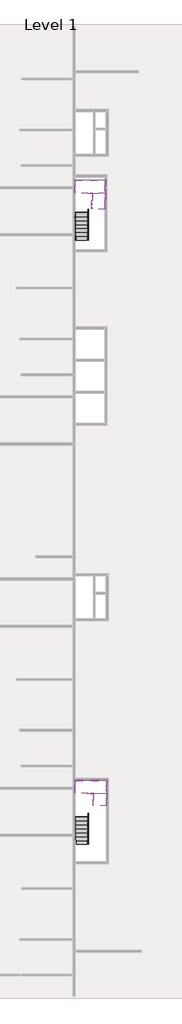
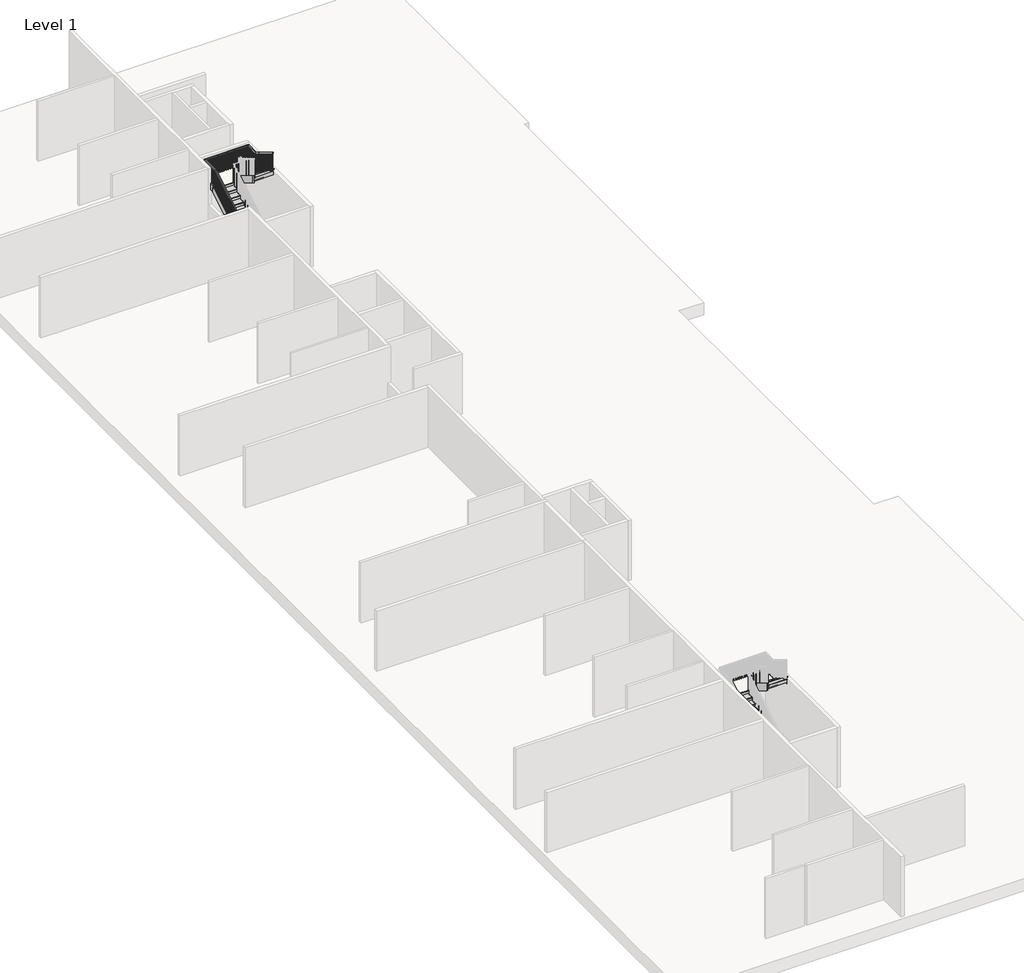
# One storey, part 8 of 8: 16 members, 4 stair flights, 2 slabs, 1 railing.
"""IFC4 building model written with IfcOpenShell, lengths in millimetres."""

from ifc_helpers import new_model, si_unit, frame, origin, place, context, project, spatial, polyline, outline, extrude, faceted_brep, transform, mapped, element, save
from components import non_monolithic_landing_1722db8f, non_monolithic_landing_351a0d85, stair_flight_df872bfd, stair_flight_7c360194, stair_flight_c0f4d4ee, stair_flight_213872ae

model = new_model("IFC4")

# Units and contexts
model_context = context("Model", 3, world=origin())
ifc_project = project(units=[si_unit("LENGTHUNIT", "METRE", prefix="MILLI")], contexts=[model_context])

# Site, building, storey
site = spatial("IfcSite", under=ifc_project)
building = spatial("IfcBuilding", under=site)
storey = spatial("IfcBuildingStorey", under=building, Name="Level 1", Elevation=25234.6172466)

# Members
placement = place(None, origin())
element("IfcMember", 1, ObjectType="Stringer - 2\" Width", at=placement, inside=storey, context=model_context, shape_type="SweptSolid", body=[
    extrude(outline(polyline([(-23154.3851539, 25234.6172466), (-23154.3851539, 25446.7317586), (-19467.0440987, 27681.4839133), (-19381.8896422, 27376.6839133), (-22916.2996422, 25234.6172466), (-23154.3851539, 25234.6172466)])), frame((-3668.2415084, 0.0, 0.0), z_axis=(1.0, 0.0, 0.0), x_axis=(0.0, 1.0, 0.0)), (0.0, 0.0, 1.0), 50.8),
])
element("IfcMember", 2, ObjectType="Stringer - 2\" Width", at=placement, inside=storey, context=model_context, shape_type="SweptSolid", body=[
    extrude(outline(polyline([(-23154.3851539, 25234.6172466), (-23154.3851539, 25446.7317586), (-19572.9851539, 27617.2772131), (-19572.9851539, 27260.8684516), (-22916.2996422, 25234.6172466), (-23154.3851539, 25234.6172466)])), frame((-2703.0415084, 0.0, 0.0), z_axis=(1.0, 0.0, 0.0), x_axis=(0.0, 1.0, 0.0)), (0.0, 0.0, 1.0), 50.8),
])
element("IfcMember", 3, ObjectType="Stringer - 2\" Width", at=placement, inside=storey, context=model_context, shape_type="SweptSolid", body=[
    extrude(outline(polyline([(-19297.9262092, 27681.4839133), (-19383.0806657, 27376.6839133), (-20360.3851539, 27968.9896637), (-20360.3851539, 28325.3984252), (-19297.9262092, 27681.4839133)])), frame((-1382.2415084, 0.0, 0.0), z_axis=(1.0, 0.0, 0.0), x_axis=(0.0, 1.0, 0.0)), (0.0, 0.0, 1.0), 50.8),
])
element("IfcMember", 4, ObjectType="Stringer - 2\" Width", at=placement, inside=storey, context=model_context, shape_type="SweptSolid", body=[
    extrude(outline(polyline([(-19522.1851539, 27817.3984252), (-19522.1851539, 27460.9896637), (-20360.3851539, 27968.9896637), (-20360.3851539, 28325.3984252), (-19522.1851539, 27817.3984252)])), frame((-2347.4415084, 0.0, 0.0), z_axis=(1.0, 0.0, 0.0), x_axis=(0.0, 1.0, 0.0)), (0.0, 0.0, 1.0), 50.8),
])
element("IfcMember", 5, ObjectType="Stringer - 2\" Width", at=placement, inside=storey, context=model_context, shape_type="Brep", body=[
    faceted_brep([(-1382.2415084, -19297.9262092, 27681.4839133), (-1331.4415084, -19297.9262092, 27681.4839133), (-1331.4415084, -18556.9851539, 27681.4839133), (-1382.2415084, -18607.7851539, 27681.4839133), (-1382.2415084, -19383.0806657, 27376.6839133), (-1382.2415084, -18607.7851539, 27376.6839133), (-1331.4415084, -19383.0806657, 27376.6839133), (-1331.4415084, -18556.9851539, 27376.6839133)], [[[0, 1, 2, 3]], [[4, 0, 3, 5]], [[6, 4, 5, 7]], [[1, 6, 7, 2]], [[1, 0, 4, 6]], [[2, 7, 5, 3]]]),
])
element("IfcMember", 6, ObjectType="Stringer - 2\" Width", at=placement, inside=storey, context=model_context, shape_type="SweptSolid", body=[
    extrude(outline(polyline([(-1331.4415084, -18556.9851539), (-1382.2415084, -18607.7851539), (-3617.4415084, -18607.7851539), (-3668.2415084, -18556.9851539), (-1331.4415084, -18556.9851539)])), frame((0.0, 0.0, 27376.6839133), z_axis=(0.0, 0.0, 1.0), x_axis=(1.0, 0.0, 0.0)), (0.0, 0.0, 1.0), 304.8),
])
element("IfcMember", 7, ObjectType="Stringer - 2\" Width", at=placement, inside=storey, context=model_context, shape_type="Brep", body=[
    faceted_brep([(-3617.4415084, -18607.7851539, 27681.4839133), (-3668.2415084, -18556.9851539, 27681.4839133), (-3668.2415084, -19467.0440987, 27681.4839133), (-3617.4415084, -19467.0440987, 27681.4839133), (-3617.4415084, -18607.7851539, 27376.6839133), (-3617.4415084, -19381.8896422, 27376.6839133), (-3668.2415084, -18556.9851539, 27376.6839133), (-3668.2415084, -19381.8896422, 27376.6839133)], [[[0, 1, 2, 3]], [[4, 0, 3, 5]], [[6, 4, 5, 7]], [[1, 6, 7, 2]], [[1, 0, 4, 6]], [[2, 7, 5, 3]]]),
])
element("IfcMember", 8, ObjectType="Stringer - 2\" Width", at=placement, inside=storey, context=model_context, shape_type="SweptSolid", body=[
    extrude(outline(polyline([(-2703.0415084, -19572.9851539), (-2703.0415084, -19522.1851539), (-2347.4415084, -19522.1851539), (-2347.4415084, -19572.9851539), (-2703.0415084, -19572.9851539)])), frame((0.0, 0.0, 27376.6839133), z_axis=(0.0, 0.0, 1.0), x_axis=(1.0, 0.0, 0.0)), (0.0, 0.0, 1.0), 304.8),
])
element("IfcMember", 9, ObjectType="Stringer - 2\" Width", at=placement, inside=storey, context=model_context, shape_type="SweptSolid", body=[
    extrude(outline(polyline([(19841.9216096, 25234.6172466), (19841.9216096, 25446.7317586), (23249.8626649, 27512.1505799), (23335.0171214, 27207.3505799), (20080.0071214, 25234.6172466), (19841.9216096, 25234.6172466)])), frame((-3668.2415084, 0.0, 0.0), z_axis=(1.0, 0.0, 0.0), x_axis=(0.0, 1.0, 0.0)), (0.0, 0.0, 1.0), 50.8),
])
element("IfcMember", 10, ObjectType="Stringer - 2\" Width", at=placement, inside=storey, context=model_context, shape_type="SweptSolid", body=[
    extrude(outline(polyline([(19841.9216096, 25234.6172466), (19841.9216096, 25446.7317586), (23143.9216096, 27447.9438798), (23143.9216096, 27091.5351183), (20080.0071214, 25234.6172466), (19841.9216096, 25234.6172466)])), frame((-2703.0415084, 0.0, 0.0), z_axis=(1.0, 0.0, 0.0), x_axis=(0.0, 1.0, 0.0)), (0.0, 0.0, 1.0), 50.8),
])
element("IfcMember", 11, ObjectType="Stringer - 2\" Width", at=placement, inside=storey, context=model_context, shape_type="SweptSolid", body=[
    extrude(outline(polyline([(23418.9805543, 27512.1505799), (23333.8260978, 27207.3505799), (22077.1216096, 27968.9896637), (22077.1216096, 28325.3984252), (23418.9805543, 27512.1505799)])), frame((-1483.8415084, 0.0, 0.0), z_axis=(1.0, 0.0, 0.0), x_axis=(0.0, 1.0, 0.0)), (0.0, 0.0, 1.0), 50.8),
])
element("IfcMember", 12, ObjectType="Stringer - 2\" Width", at=placement, inside=storey, context=model_context, shape_type="SweptSolid", body=[
    extrude(outline(polyline([(23194.7216096, 27648.0650919), (23194.7216096, 27291.6563304), (22077.1216096, 27968.9896637), (22077.1216096, 28325.3984252), (23194.7216096, 27648.0650919)])), frame((-2449.0415084, 0.0, 0.0), z_axis=(1.0, 0.0, 0.0), x_axis=(0.0, 1.0, 0.0)), (0.0, 0.0, 1.0), 50.8),
])
element("IfcMember", 13, ObjectType="Stringer - 2\" Width", at=placement, inside=storey, context=model_context, shape_type="Brep", body=[
    faceted_brep([(-1483.8415084, 23418.9805543, 27512.1505799), (-1433.0415084, 23418.9805543, 27512.1505799), (-1433.0415084, 24159.9216096, 27512.1505799), (-1483.8415084, 24109.1216096, 27512.1505799), (-1483.8415084, 23333.8260978, 27207.3505799), (-1483.8415084, 24109.1216096, 27207.3505799), (-1433.0415084, 23333.8260978, 27207.3505799), (-1433.0415084, 24159.9216096, 27207.3505799)], [[[0, 1, 2, 3]], [[4, 0, 3, 5]], [[6, 4, 5, 7]], [[1, 6, 7, 2]], [[1, 0, 4, 6]], [[2, 7, 5, 3]]]),
])
element("IfcMember", 14, ObjectType="Stringer - 2\" Width", at=placement, inside=storey, context=model_context, shape_type="SweptSolid", body=[
    extrude(outline(polyline([(-1433.0415084, 24159.9216096), (-1483.8415084, 24109.1216096), (-3617.4415084, 24109.1216096), (-3668.2415084, 24159.9216096), (-1433.0415084, 24159.9216096)])), frame((0.0, 0.0, 27207.3505799), z_axis=(0.0, 0.0, 1.0), x_axis=(1.0, 0.0, 0.0)), (0.0, 0.0, 1.0), 304.8),
])
element("IfcMember", 15, ObjectType="Stringer - 2\" Width", at=placement, inside=storey, context=model_context, shape_type="Brep", body=[
    faceted_brep([(-3617.4415084, 24109.1216096, 27512.1505799), (-3668.2415084, 24159.9216096, 27512.1505799), (-3668.2415084, 23249.8626649, 27512.1505799), (-3617.4415084, 23249.8626649, 27512.1505799), (-3617.4415084, 24109.1216096, 27207.3505799), (-3617.4415084, 23335.0171214, 27207.3505799), (-3668.2415084, 24159.9216096, 27207.3505799), (-3668.2415084, 23335.0171214, 27207.3505799)], [[[0, 1, 2, 3]], [[4, 0, 3, 5]], [[6, 4, 5, 7]], [[1, 6, 7, 2]], [[1, 0, 4, 6]], [[2, 7, 5, 3]]]),
])
element("IfcMember", 16, ObjectType="Stringer - 2\" Width", at=placement, inside=storey, context=model_context, shape_type="SweptSolid", body=[
    extrude(outline(polyline([(-2703.0415084, 23143.9216096), (-2703.0415084, 23194.7216096), (-2449.0415084, 23194.7216096), (-2449.0415084, 23143.9216096), (-2703.0415084, 23143.9216096)])), frame((0.0, 0.0, 27207.3505799), z_axis=(0.0, 0.0, 1.0), x_axis=(1.0, 0.0, 0.0)), (0.0, 0.0, 1.0), 304.8),
])

# Railing
element("IfcRailing", 17, ObjectType="Handrail - Rectangular", at=placement, inside=storey, context=model_context, shape_type="SolidModel", body=[
    faceted_brep([(-3617.4415084, 19841.9216096, 26318.3505799), (-3617.4415084, 19841.9216096, 26258.9491197), (-3566.6415084, 19841.9216096, 26258.9491197), (-3566.6415084, 19841.9216096, 26318.3505799), (-3617.4415084, 23194.7216096, 28350.3505799), (-3617.4415084, 23208.914019, 28299.5505799), (-3566.6415084, 23208.914019, 28299.5505799), (-3566.6415084, 23194.7216096, 28350.3505799), (-3617.4415084, 24109.1216096, 28350.3505799), (-3617.4415084, 24109.1216096, 28299.5505799), (-3566.6415084, 24058.3216096, 28299.5505799), (-3566.6415084, 24058.3216096, 28350.3505799), (-1483.8415084, 24109.1216096, 28350.3505799), (-1483.8415084, 24109.1216096, 28299.5505799), (-1534.6415084, 24058.3216096, 28299.5505799), (-1534.6415084, 24058.3216096, 28350.3505799), (-1483.8415084, 23474.1216096, 28350.3505799), (-1483.8415084, 23459.9292002, 28299.5505799), (-1534.6415084, 23459.9292002, 28299.5505799), (-1534.6415084, 23474.1216096, 28350.3505799), (-1483.8415084, 23194.7216096, 28519.6839133), (-1483.8415084, 23168.3918824, 28476.2398634), (-1534.6415084, 23168.3918824, 28476.2398634), (-1534.6415084, 23194.7216096, 28519.6839133), (-1483.8415084, 22077.1216096, 29197.0172466), (-1534.6415084, 22077.1216096, 29197.0172466), (-1534.6415084, 22077.1216096, 29137.6157863), (-1483.8415084, 22077.1216096, 29137.6157863)], [[[0, 1, 2, 3]], [[1, 0, 4, 5]], [[2, 1, 5, 6]], [[3, 2, 6, 7]], [[0, 3, 7, 4]], [[5, 4, 8, 9]], [[6, 5, 9, 10]], [[7, 6, 10, 11]], [[4, 7, 11, 8]], [[9, 8, 12, 13]], [[10, 9, 13, 14]], [[11, 10, 14, 15]], [[8, 11, 15, 12]], [[13, 12, 16, 17]], [[14, 13, 17, 18]], [[15, 14, 18, 19]], [[12, 15, 19, 16]], [[17, 16, 20, 21]], [[18, 17, 21, 22]], [[19, 18, 22, 23]], [[16, 19, 23, 20]], [[24, 25, 26, 27]], [[21, 20, 24, 27]], [[22, 21, 27, 26]], [[23, 22, 26, 25]], [[20, 23, 25, 24]]]),
    extrude(outline(polyline([(22188.2466096, 29070.2673015), (22188.2466096, 28113.2839133), (22169.1966096, 28113.2839133), (22169.1966096, 29081.812756), (22188.2466096, 29070.2673015)])), frame((-1518.7665084, 0.0, 0.0), z_axis=(1.0, 0.0, 0.0), x_axis=(0.0, 1.0, 0.0)), (0.0, 0.0, 1.0), 19.05),
    extrude(outline(polyline([(22289.8466096, 29008.6915439), (22289.8466096, 28113.2839133), (22270.7966096, 28113.2839133), (22270.7966096, 29020.2369985), (22289.8466096, 29008.6915439)])), frame((-1518.7665084, 0.0, 0.0), z_axis=(1.0, 0.0, 0.0), x_axis=(0.0, 1.0, 0.0)), (0.0, 0.0, 1.0), 19.05),
    extrude(outline(polyline([(22391.4466096, 28947.1157863), (22391.4466096, 27943.9505799), (22372.3966096, 27943.9505799), (22372.3966096, 28958.6612409), (22391.4466096, 28947.1157863)])), frame((-1518.7665084, 0.0, 0.0), z_axis=(1.0, 0.0, 0.0), x_axis=(0.0, 1.0, 0.0)), (0.0, 0.0, 1.0), 19.05),
    extrude(outline(polyline([(22493.0466096, 28885.5400288), (22493.0466096, 27943.9505799), (22473.9966096, 27943.9505799), (22473.9966096, 28897.0854833), (22493.0466096, 28885.5400288)])), frame((-1518.7665084, 0.0, 0.0), z_axis=(1.0, 0.0, 0.0), x_axis=(0.0, 1.0, 0.0)), (0.0, 0.0, 1.0), 19.05),
    extrude(outline(polyline([(22594.6466096, 28823.9642712), (22594.6466096, 27943.9505799), (22575.5966096, 27943.9505799), (22575.5966096, 28835.5097257), (22594.6466096, 28823.9642712)])), frame((-1518.7665084, 0.0, 0.0), z_axis=(1.0, 0.0, 0.0), x_axis=(0.0, 1.0, 0.0)), (0.0, 0.0, 1.0), 19.05),
    extrude(outline(polyline([(22696.2466096, 28762.3885136), (22696.2466096, 27774.6172466), (22677.1966096, 27774.6172466), (22677.1966096, 28773.9339682), (22696.2466096, 28762.3885136)])), frame((-1518.7665084, 0.0, 0.0), z_axis=(1.0, 0.0, 0.0), x_axis=(0.0, 1.0, 0.0)), (0.0, 0.0, 1.0), 19.05),
    extrude(outline(polyline([(22797.8466096, 28700.812756), (22797.8466096, 27774.6172466), (22778.7966096, 27774.6172466), (22778.7966096, 28712.3582106), (22797.8466096, 28700.812756)])), frame((-1518.7665084, 0.0, 0.0), z_axis=(1.0, 0.0, 0.0), x_axis=(0.0, 1.0, 0.0)), (0.0, 0.0, 1.0), 19.05),
    extrude(outline(polyline([(22899.4466096, 28639.2369985), (22899.4466096, 27774.6172466), (22880.3966096, 27774.6172466), (22880.3966096, 28650.782453), (22899.4466096, 28639.2369985)])), frame((-1518.7665084, 0.0, 0.0), z_axis=(1.0, 0.0, 0.0), x_axis=(0.0, 1.0, 0.0)), (0.0, 0.0, 1.0), 19.05),
    extrude(outline(polyline([(23001.0466096, 28577.6612409), (23001.0466096, 27605.2839133), (22981.9966096, 27605.2839133), (22981.9966096, 28589.2066954), (23001.0466096, 28577.6612409)])), frame((-1518.7665084, 0.0, 0.0), z_axis=(1.0, 0.0, 0.0), x_axis=(0.0, 1.0, 0.0)), (0.0, 0.0, 1.0), 19.05),
    extrude(outline(polyline([(23102.6466096, 28516.0854833), (23102.6466096, 27605.2839133), (23083.5966096, 27605.2839133), (23083.5966096, 28527.6309379), (23102.6466096, 28516.0854833)])), frame((-1518.7665084, 0.0, 0.0), z_axis=(1.0, 0.0, 0.0), x_axis=(0.0, 1.0, 0.0)), (0.0, 0.0, 1.0), 19.05),
    extrude(outline(polyline([(23280.4466096, 28408.3279076), (23280.4466096, 27435.9505799), (23261.3966096, 27435.9505799), (23261.3966096, 28419.8733621), (23280.4466096, 28408.3279076)])), frame((-1518.7665084, 0.0, 0.0), z_axis=(1.0, 0.0, 0.0), x_axis=(0.0, 1.0, 0.0)), (0.0, 0.0, 1.0), 19.05),
    extrude(outline(polyline([(23382.0466096, 28346.75215), (23382.0466096, 27435.9505799), (23362.9966096, 27435.9505799), (23362.9966096, 28358.2976045), (23382.0466096, 28346.75215)])), frame((-1518.7665084, 0.0, 0.0), z_axis=(1.0, 0.0, 0.0), x_axis=(0.0, 1.0, 0.0)), (0.0, 0.0, 1.0), 19.05),
    extrude(outline(polyline([(-1499.7165084, 23483.6466096), (-1499.7165084, 23464.5966096), (-1518.7665084, 23464.5966096), (-1518.7665084, 23483.6466096), (-1499.7165084, 23483.6466096)])), frame((0.0, 0.0, 27435.9505799), z_axis=(0.0, 0.0, 1.0), x_axis=(1.0, 0.0, 0.0)), (0.0, 0.0, 1.0), 863.6),
    extrude(outline(polyline([(-1499.7165084, 23585.2466096), (-1499.7165084, 23566.1966096), (-1518.7665084, 23566.1966096), (-1518.7665084, 23585.2466096), (-1499.7165084, 23585.2466096)])), frame((0.0, 0.0, 27435.9505799), z_axis=(0.0, 0.0, 1.0), x_axis=(1.0, 0.0, 0.0)), (0.0, 0.0, 1.0), 863.6),
    extrude(outline(polyline([(-1499.7165084, 23686.8466096), (-1499.7165084, 23667.7966096), (-1518.7665084, 23667.7966096), (-1518.7665084, 23686.8466096), (-1499.7165084, 23686.8466096)])), frame((0.0, 0.0, 27435.9505799), z_axis=(0.0, 0.0, 1.0), x_axis=(1.0, 0.0, 0.0)), (0.0, 0.0, 1.0), 863.6),
    extrude(outline(polyline([(-1499.7165084, 23788.4466096), (-1499.7165084, 23769.3966096), (-1518.7665084, 23769.3966096), (-1518.7665084, 23788.4466096), (-1499.7165084, 23788.4466096)])), frame((0.0, 0.0, 27435.9505799), z_axis=(0.0, 0.0, 1.0), x_axis=(1.0, 0.0, 0.0)), (0.0, 0.0, 1.0), 863.6),
    extrude(outline(polyline([(-1499.7165084, 23890.0466096), (-1499.7165084, 23870.9966096), (-1518.7665084, 23870.9966096), (-1518.7665084, 23890.0466096), (-1499.7165084, 23890.0466096)])), frame((0.0, 0.0, 27435.9505799), z_axis=(0.0, 0.0, 1.0), x_axis=(1.0, 0.0, 0.0)), (0.0, 0.0, 1.0), 863.6),
    extrude(outline(polyline([(-1499.7165084, 23991.6466096), (-1499.7165084, 23972.5966096), (-1518.7665084, 23972.5966096), (-1518.7665084, 23991.6466096), (-1499.7165084, 23991.6466096)])), frame((0.0, 0.0, 27435.9505799), z_axis=(0.0, 0.0, 1.0), x_axis=(1.0, 0.0, 0.0)), (0.0, 0.0, 1.0), 863.6),
    extrude(outline(polyline([(-1569.5665084, 24093.2466096), (-1550.5165084, 24093.2466096), (-1550.5165084, 24074.1966096), (-1569.5665084, 24074.1966096), (-1569.5665084, 24093.2466096)])), frame((0.0, 0.0, 27435.9505799), z_axis=(0.0, 0.0, 1.0), x_axis=(1.0, 0.0, 0.0)), (0.0, 0.0, 1.0), 863.6),
    extrude(outline(polyline([(-1671.1665084, 24093.2466096), (-1652.1165084, 24093.2466096), (-1652.1165084, 24074.1966096), (-1671.1665084, 24074.1966096), (-1671.1665084, 24093.2466096)])), frame((0.0, 0.0, 27435.9505799), z_axis=(0.0, 0.0, 1.0), x_axis=(1.0, 0.0, 0.0)), (0.0, 0.0, 1.0), 863.6),
    extrude(outline(polyline([(-1772.7665084, 24093.2466096), (-1753.7165084, 24093.2466096), (-1753.7165084, 24074.1966096), (-1772.7665084, 24074.1966096), (-1772.7665084, 24093.2466096)])), frame((0.0, 0.0, 27435.9505799), z_axis=(0.0, 0.0, 1.0), x_axis=(1.0, 0.0, 0.0)), (0.0, 0.0, 1.0), 863.6),
    extrude(outline(polyline([(-1874.3665084, 24093.2466096), (-1855.3165084, 24093.2466096), (-1855.3165084, 24074.1966096), (-1874.3665084, 24074.1966096), (-1874.3665084, 24093.2466096)])), frame((0.0, 0.0, 27435.9505799), z_axis=(0.0, 0.0, 1.0), x_axis=(1.0, 0.0, 0.0)), (0.0, 0.0, 1.0), 863.6),
    extrude(outline(polyline([(-1975.9665084, 24093.2466096), (-1956.9165084, 24093.2466096), (-1956.9165084, 24074.1966096), (-1975.9665084, 24074.1966096), (-1975.9665084, 24093.2466096)])), frame((0.0, 0.0, 27435.9505799), z_axis=(0.0, 0.0, 1.0), x_axis=(1.0, 0.0, 0.0)), (0.0, 0.0, 1.0), 863.6),
    extrude(outline(polyline([(-2077.5665084, 24093.2466096), (-2058.5165084, 24093.2466096), (-2058.5165084, 24074.1966096), (-2077.5665084, 24074.1966096), (-2077.5665084, 24093.2466096)])), frame((0.0, 0.0, 27435.9505799), z_axis=(0.0, 0.0, 1.0), x_axis=(1.0, 0.0, 0.0)), (0.0, 0.0, 1.0), 863.6),
    extrude(outline(polyline([(-2179.1665084, 24093.2466096), (-2160.1165084, 24093.2466096), (-2160.1165084, 24074.1966096), (-2179.1665084, 24074.1966096), (-2179.1665084, 24093.2466096)])), frame((0.0, 0.0, 27435.9505799), z_axis=(0.0, 0.0, 1.0), x_axis=(1.0, 0.0, 0.0)), (0.0, 0.0, 1.0), 863.6),
    extrude(outline(polyline([(-2280.7665084, 24093.2466096), (-2261.7165084, 24093.2466096), (-2261.7165084, 24074.1966096), (-2280.7665084, 24074.1966096), (-2280.7665084, 24093.2466096)])), frame((0.0, 0.0, 27435.9505799), z_axis=(0.0, 0.0, 1.0), x_axis=(1.0, 0.0, 0.0)), (0.0, 0.0, 1.0), 863.6),
    extrude(outline(polyline([(-2382.3665084, 24093.2466096), (-2363.3165084, 24093.2466096), (-2363.3165084, 24074.1966096), (-2382.3665084, 24074.1966096), (-2382.3665084, 24093.2466096)])), frame((0.0, 0.0, 27435.9505799), z_axis=(0.0, 0.0, 1.0), x_axis=(1.0, 0.0, 0.0)), (0.0, 0.0, 1.0), 863.6),
    extrude(outline(polyline([(-2483.9665084, 24093.2466096), (-2464.9165084, 24093.2466096), (-2464.9165084, 24074.1966096), (-2483.9665084, 24074.1966096), (-2483.9665084, 24093.2466096)])), frame((0.0, 0.0, 27435.9505799), z_axis=(0.0, 0.0, 1.0), x_axis=(1.0, 0.0, 0.0)), (0.0, 0.0, 1.0), 863.6),
    extrude(outline(polyline([(-2585.5665084, 24093.2466096), (-2566.5165084, 24093.2466096), (-2566.5165084, 24074.1966096), (-2585.5665084, 24074.1966096), (-2585.5665084, 24093.2466096)])), frame((0.0, 0.0, 27435.9505799), z_axis=(0.0, 0.0, 1.0), x_axis=(1.0, 0.0, 0.0)), (0.0, 0.0, 1.0), 863.6),
    extrude(outline(polyline([(-2687.1665084, 24093.2466096), (-2668.1165084, 24093.2466096), (-2668.1165084, 24074.1966096), (-2687.1665084, 24074.1966096), (-2687.1665084, 24093.2466096)])), frame((0.0, 0.0, 27435.9505799), z_axis=(0.0, 0.0, 1.0), x_axis=(1.0, 0.0, 0.0)), (0.0, 0.0, 1.0), 863.6),
    extrude(outline(polyline([(-2788.7665084, 24093.2466096), (-2769.7165084, 24093.2466096), (-2769.7165084, 24074.1966096), (-2788.7665084, 24074.1966096), (-2788.7665084, 24093.2466096)])), frame((0.0, 0.0, 27435.9505799), z_axis=(0.0, 0.0, 1.0), x_axis=(1.0, 0.0, 0.0)), (0.0, 0.0, 1.0), 863.6),
    extrude(outline(polyline([(-2890.3665084, 24093.2466096), (-2871.3165084, 24093.2466096), (-2871.3165084, 24074.1966096), (-2890.3665084, 24074.1966096), (-2890.3665084, 24093.2466096)])), frame((0.0, 0.0, 27435.9505799), z_axis=(0.0, 0.0, 1.0), x_axis=(1.0, 0.0, 0.0)), (0.0, 0.0, 1.0), 863.6),
    extrude(outline(polyline([(-2991.9665084, 24093.2466096), (-2972.9165084, 24093.2466096), (-2972.9165084, 24074.1966096), (-2991.9665084, 24074.1966096), (-2991.9665084, 24093.2466096)])), frame((0.0, 0.0, 27435.9505799), z_axis=(0.0, 0.0, 1.0), x_axis=(1.0, 0.0, 0.0)), (0.0, 0.0, 1.0), 863.6),
    extrude(outline(polyline([(-3093.5665084, 24093.2466096), (-3074.5165084, 24093.2466096), (-3074.5165084, 24074.1966096), (-3093.5665084, 24074.1966096), (-3093.5665084, 24093.2466096)])), frame((0.0, 0.0, 27435.9505799), z_axis=(0.0, 0.0, 1.0), x_axis=(1.0, 0.0, 0.0)), (0.0, 0.0, 1.0), 863.6),
    extrude(outline(polyline([(-3195.1665084, 24093.2466096), (-3176.1165084, 24093.2466096), (-3176.1165084, 24074.1966096), (-3195.1665084, 24074.1966096), (-3195.1665084, 24093.2466096)])), frame((0.0, 0.0, 27435.9505799), z_axis=(0.0, 0.0, 1.0), x_axis=(1.0, 0.0, 0.0)), (0.0, 0.0, 1.0), 863.6),
    extrude(outline(polyline([(-3296.7665084, 24093.2466096), (-3277.7165084, 24093.2466096), (-3277.7165084, 24074.1966096), (-3296.7665084, 24074.1966096), (-3296.7665084, 24093.2466096)])), frame((0.0, 0.0, 27435.9505799), z_axis=(0.0, 0.0, 1.0), x_axis=(1.0, 0.0, 0.0)), (0.0, 0.0, 1.0), 863.6),
    extrude(outline(polyline([(-3398.3665084, 24093.2466096), (-3379.3165084, 24093.2466096), (-3379.3165084, 24074.1966096), (-3398.3665084, 24074.1966096), (-3398.3665084, 24093.2466096)])), frame((0.0, 0.0, 27435.9505799), z_axis=(0.0, 0.0, 1.0), x_axis=(1.0, 0.0, 0.0)), (0.0, 0.0, 1.0), 863.6),
    extrude(outline(polyline([(-3499.9665084, 24093.2466096), (-3480.9165084, 24093.2466096), (-3480.9165084, 24074.1966096), (-3499.9665084, 24074.1966096), (-3499.9665084, 24093.2466096)])), frame((0.0, 0.0, 27435.9505799), z_axis=(0.0, 0.0, 1.0), x_axis=(1.0, 0.0, 0.0)), (0.0, 0.0, 1.0), 863.6),
    extrude(outline(polyline([(-3601.5665084, 23997.9966096), (-3601.5665084, 24017.0466096), (-3582.5165084, 24017.0466096), (-3582.5165084, 23997.9966096), (-3601.5665084, 23997.9966096)])), frame((0.0, 0.0, 27435.9505799), z_axis=(0.0, 0.0, 1.0), x_axis=(1.0, 0.0, 0.0)), (0.0, 0.0, 1.0), 863.6),
    extrude(outline(polyline([(-3601.5665084, 23896.3966096), (-3601.5665084, 23915.4466096), (-3582.5165084, 23915.4466096), (-3582.5165084, 23896.3966096), (-3601.5665084, 23896.3966096)])), frame((0.0, 0.0, 27435.9505799), z_axis=(0.0, 0.0, 1.0), x_axis=(1.0, 0.0, 0.0)), (0.0, 0.0, 1.0), 863.6),
    extrude(outline(polyline([(-3601.5665084, 23794.7966096), (-3601.5665084, 23813.8466096), (-3582.5165084, 23813.8466096), (-3582.5165084, 23794.7966096), (-3601.5665084, 23794.7966096)])), frame((0.0, 0.0, 27435.9505799), z_axis=(0.0, 0.0, 1.0), x_axis=(1.0, 0.0, 0.0)), (0.0, 0.0, 1.0), 863.6),
    extrude(outline(polyline([(-3601.5665084, 23693.1966096), (-3601.5665084, 23712.2466096), (-3582.5165084, 23712.2466096), (-3582.5165084, 23693.1966096), (-3601.5665084, 23693.1966096)])), frame((0.0, 0.0, 27435.9505799), z_axis=(0.0, 0.0, 1.0), x_axis=(1.0, 0.0, 0.0)), (0.0, 0.0, 1.0), 863.6),
    extrude(outline(polyline([(-3601.5665084, 23591.5966096), (-3601.5665084, 23610.6466096), (-3582.5165084, 23610.6466096), (-3582.5165084, 23591.5966096), (-3601.5665084, 23591.5966096)])), frame((0.0, 0.0, 27435.9505799), z_axis=(0.0, 0.0, 1.0), x_axis=(1.0, 0.0, 0.0)), (0.0, 0.0, 1.0), 863.6),
    extrude(outline(polyline([(-3601.5665084, 23489.9966096), (-3601.5665084, 23509.0466096), (-3582.5165084, 23509.0466096), (-3582.5165084, 23489.9966096), (-3601.5665084, 23489.9966096)])), frame((0.0, 0.0, 27435.9505799), z_axis=(0.0, 0.0, 1.0), x_axis=(1.0, 0.0, 0.0)), (0.0, 0.0, 1.0), 863.6),
    extrude(outline(polyline([(-3601.5665084, 23388.3966096), (-3601.5665084, 23407.4466096), (-3582.5165084, 23407.4466096), (-3582.5165084, 23388.3966096), (-3601.5665084, 23388.3966096)])), frame((0.0, 0.0, 27435.9505799), z_axis=(0.0, 0.0, 1.0), x_axis=(1.0, 0.0, 0.0)), (0.0, 0.0, 1.0), 863.6),
    extrude(outline(polyline([(-3601.5665084, 23286.7966096), (-3601.5665084, 23305.8466096), (-3582.5165084, 23305.8466096), (-3582.5165084, 23286.7966096), (-3601.5665084, 23286.7966096)])), frame((0.0, 0.0, 27435.9505799), z_axis=(0.0, 0.0, 1.0), x_axis=(1.0, 0.0, 0.0)), (0.0, 0.0, 1.0), 863.6),
    extrude(outline(polyline([(23102.6466096, 28235.1460894), (23102.6466096, 27266.6172466), (23083.5966096, 27266.6172466), (23083.5966096, 28223.6006348), (23102.6466096, 28235.1460894)])), frame((-3601.5665084, 0.0, 0.0), z_axis=(1.0, 0.0, 0.0), x_axis=(0.0, 1.0, 0.0)), (0.0, 0.0, 1.0), 19.05),
    extrude(outline(polyline([(23001.0466096, 28173.5703318), (23001.0466096, 27266.6172466), (22981.9966096, 27266.6172466), (22981.9966096, 28162.0248773), (23001.0466096, 28173.5703318)])), frame((-3601.5665084, 0.0, 0.0), z_axis=(1.0, 0.0, 0.0), x_axis=(0.0, 1.0, 0.0)), (0.0, 0.0, 1.0), 19.05),
    extrude(outline(polyline([(22899.4466096, 28111.9945742), (22899.4466096, 27097.2839133), (22880.3966096, 27097.2839133), (22880.3966096, 28100.4491197), (22899.4466096, 28111.9945742)])), frame((-3601.5665084, 0.0, 0.0), z_axis=(1.0, 0.0, 0.0), x_axis=(0.0, 1.0, 0.0)), (0.0, 0.0, 1.0), 19.05),
    extrude(outline(polyline([(22797.8466096, 28050.4188167), (22797.8466096, 27097.2839133), (22778.7966096, 27097.2839133), (22778.7966096, 28038.8733621), (22797.8466096, 28050.4188167)])), frame((-3601.5665084, 0.0, 0.0), z_axis=(1.0, 0.0, 0.0), x_axis=(0.0, 1.0, 0.0)), (0.0, 0.0, 1.0), 19.05),
    extrude(outline(polyline([(22696.2466096, 27988.8430591), (22696.2466096, 27097.2839133), (22677.1966096, 27097.2839133), (22677.1966096, 27977.2976045), (22696.2466096, 27988.8430591)])), frame((-3601.5665084, 0.0, 0.0), z_axis=(1.0, 0.0, 0.0), x_axis=(0.0, 1.0, 0.0)), (0.0, 0.0, 1.0), 19.05),
    extrude(outline(polyline([(22594.6466096, 27927.2673015), (22594.6466096, 26927.9505799), (22575.5966096, 26927.9505799), (22575.5966096, 27915.721847), (22594.6466096, 27927.2673015)])), frame((-3601.5665084, 0.0, 0.0), z_axis=(1.0, 0.0, 0.0), x_axis=(0.0, 1.0, 0.0)), (0.0, 0.0, 1.0), 19.05),
    extrude(outline(polyline([(22493.0466096, 27865.6915439), (22493.0466096, 26927.9505799), (22473.9966096, 26927.9505799), (22473.9966096, 27854.1460894), (22493.0466096, 27865.6915439)])), frame((-3601.5665084, 0.0, 0.0), z_axis=(1.0, 0.0, 0.0), x_axis=(0.0, 1.0, 0.0)), (0.0, 0.0, 1.0), 19.05),
    extrude(outline(polyline([(22391.4466096, 27804.1157863), (22391.4466096, 26927.9505799), (22372.3966096, 26927.9505799), (22372.3966096, 27792.5703318), (22391.4466096, 27804.1157863)])), frame((-3601.5665084, 0.0, 0.0), z_axis=(1.0, 0.0, 0.0), x_axis=(0.0, 1.0, 0.0)), (0.0, 0.0, 1.0), 19.05),
    extrude(outline(polyline([(22289.8466096, 27742.5400288), (22289.8466096, 26758.6172466), (22270.7966096, 26758.6172466), (22270.7966096, 27730.9945742), (22289.8466096, 27742.5400288)])), frame((-3601.5665084, 0.0, 0.0), z_axis=(1.0, 0.0, 0.0), x_axis=(0.0, 1.0, 0.0)), (0.0, 0.0, 1.0), 19.05),
    extrude(outline(polyline([(22188.2466096, 27680.9642712), (22188.2466096, 26758.6172466), (22169.1966096, 26758.6172466), (22169.1966096, 27669.4188167), (22188.2466096, 27680.9642712)])), frame((-3601.5665084, 0.0, 0.0), z_axis=(1.0, 0.0, 0.0), x_axis=(0.0, 1.0, 0.0)), (0.0, 0.0, 1.0), 19.05),
    extrude(outline(polyline([(22086.6466096, 27619.3885136), (22086.6466096, 26758.6172466), (22067.5966096, 26758.6172466), (22067.5966096, 27607.8430591), (22086.6466096, 27619.3885136)])), frame((-3601.5665084, 0.0, 0.0), z_axis=(1.0, 0.0, 0.0), x_axis=(0.0, 1.0, 0.0)), (0.0, 0.0, 1.0), 19.05),
    extrude(outline(polyline([(21985.0466096, 27557.812756), (21985.0466096, 26589.2839133), (21965.9966096, 26589.2839133), (21965.9966096, 27546.2673015), (21985.0466096, 27557.812756)])), frame((-3601.5665084, 0.0, 0.0), z_axis=(1.0, 0.0, 0.0), x_axis=(0.0, 1.0, 0.0)), (0.0, 0.0, 1.0), 19.05),
    extrude(outline(polyline([(21883.4466096, 27496.2369985), (21883.4466096, 26589.2839133), (21864.3966096, 26589.2839133), (21864.3966096, 27484.6915439), (21883.4466096, 27496.2369985)])), frame((-3601.5665084, 0.0, 0.0), z_axis=(1.0, 0.0, 0.0), x_axis=(0.0, 1.0, 0.0)), (0.0, 0.0, 1.0), 19.05),
    extrude(outline(polyline([(21781.8466096, 27434.6612409), (21781.8466096, 26419.9505799), (21762.7966096, 26419.9505799), (21762.7966096, 27423.1157863), (21781.8466096, 27434.6612409)])), frame((-3601.5665084, 0.0, 0.0), z_axis=(1.0, 0.0, 0.0), x_axis=(0.0, 1.0, 0.0)), (0.0, 0.0, 1.0), 19.05),
    extrude(outline(polyline([(21680.2466096, 27373.0854833), (21680.2466096, 26419.9505799), (21661.1966096, 26419.9505799), (21661.1966096, 27361.5400288), (21680.2466096, 27373.0854833)])), frame((-3601.5665084, 0.0, 0.0), z_axis=(1.0, 0.0, 0.0), x_axis=(0.0, 1.0, 0.0)), (0.0, 0.0, 1.0), 19.05),
    extrude(outline(polyline([(21578.6466096, 27311.5097257), (21578.6466096, 26419.9505799), (21559.5966096, 26419.9505799), (21559.5966096, 27299.9642712), (21578.6466096, 27311.5097257)])), frame((-3601.5665084, 0.0, 0.0), z_axis=(1.0, 0.0, 0.0), x_axis=(0.0, 1.0, 0.0)), (0.0, 0.0, 1.0), 19.05),
    extrude(outline(polyline([(21477.0466096, 27249.9339682), (21477.0466096, 26250.6172466), (21457.9966096, 26250.6172466), (21457.9966096, 27238.3885136), (21477.0466096, 27249.9339682)])), frame((-3601.5665084, 0.0, 0.0), z_axis=(1.0, 0.0, 0.0), x_axis=(0.0, 1.0, 0.0)), (0.0, 0.0, 1.0), 19.05),
    extrude(outline(polyline([(21375.4466096, 27188.3582106), (21375.4466096, 26250.6172466), (21356.3966096, 26250.6172466), (21356.3966096, 27176.812756), (21375.4466096, 27188.3582106)])), frame((-3601.5665084, 0.0, 0.0), z_axis=(1.0, 0.0, 0.0), x_axis=(0.0, 1.0, 0.0)), (0.0, 0.0, 1.0), 19.05),
    extrude(outline(polyline([(21273.8466096, 27126.782453), (21273.8466096, 26250.6172466), (21254.7966096, 26250.6172466), (21254.7966096, 27115.2369985), (21273.8466096, 27126.782453)])), frame((-3601.5665084, 0.0, 0.0), z_axis=(1.0, 0.0, 0.0), x_axis=(0.0, 1.0, 0.0)), (0.0, 0.0, 1.0), 19.05),
    extrude(outline(polyline([(21172.2466096, 27065.2066954), (21172.2466096, 26081.2839133), (21153.1966096, 26081.2839133), (21153.1966096, 27053.6612409), (21172.2466096, 27065.2066954)])), frame((-3601.5665084, 0.0, 0.0), z_axis=(1.0, 0.0, 0.0), x_axis=(0.0, 1.0, 0.0)), (0.0, 0.0, 1.0), 19.05),
    extrude(outline(polyline([(21070.6466096, 27003.6309379), (21070.6466096, 26081.2839133), (21051.5966096, 26081.2839133), (21051.5966096, 26992.0854833), (21070.6466096, 27003.6309379)])), frame((-3601.5665084, 0.0, 0.0), z_axis=(1.0, 0.0, 0.0), x_axis=(0.0, 1.0, 0.0)), (0.0, 0.0, 1.0), 19.05),
    extrude(outline(polyline([(20969.0466096, 26942.0551803), (20969.0466096, 26081.2839133), (20949.9966096, 26081.2839133), (20949.9966096, 26930.5097257), (20969.0466096, 26942.0551803)])), frame((-3601.5665084, 0.0, 0.0), z_axis=(1.0, 0.0, 0.0), x_axis=(0.0, 1.0, 0.0)), (0.0, 0.0, 1.0), 19.05),
    extrude(outline(polyline([(20867.4466096, 26880.4794227), (20867.4466096, 25911.9505799), (20848.3966096, 25911.9505799), (20848.3966096, 26868.9339682), (20867.4466096, 26880.4794227)])), frame((-3601.5665084, 0.0, 0.0), z_axis=(1.0, 0.0, 0.0), x_axis=(0.0, 1.0, 0.0)), (0.0, 0.0, 1.0), 19.05),
    extrude(outline(polyline([(20765.8466096, 26818.9036651), (20765.8466096, 25911.9505799), (20746.7966096, 25911.9505799), (20746.7966096, 26807.3582106), (20765.8466096, 26818.9036651)])), frame((-3601.5665084, 0.0, 0.0), z_axis=(1.0, 0.0, 0.0), x_axis=(0.0, 1.0, 0.0)), (0.0, 0.0, 1.0), 19.05),
    extrude(outline(polyline([(20664.2466096, 26757.3279076), (20664.2466096, 25742.6172466), (20645.1966096, 25742.6172466), (20645.1966096, 26745.782453), (20664.2466096, 26757.3279076)])), frame((-3601.5665084, 0.0, 0.0), z_axis=(1.0, 0.0, 0.0), x_axis=(0.0, 1.0, 0.0)), (0.0, 0.0, 1.0), 19.05),
    extrude(outline(polyline([(20562.6466096, 26695.75215), (20562.6466096, 25742.6172466), (20543.5966096, 25742.6172466), (20543.5966096, 26684.2066954), (20562.6466096, 26695.75215)])), frame((-3601.5665084, 0.0, 0.0), z_axis=(1.0, 0.0, 0.0), x_axis=(0.0, 1.0, 0.0)), (0.0, 0.0, 1.0), 19.05),
    extrude(outline(polyline([(20461.0466096, 26634.1763924), (20461.0466096, 25742.6172466), (20441.9966096, 25742.6172466), (20441.9966096, 26622.6309379), (20461.0466096, 26634.1763924)])), frame((-3601.5665084, 0.0, 0.0), z_axis=(1.0, 0.0, 0.0), x_axis=(0.0, 1.0, 0.0)), (0.0, 0.0, 1.0), 19.05),
    extrude(outline(polyline([(20359.4466096, 26572.6006348), (20359.4466096, 25573.2839133), (20340.3966096, 25573.2839133), (20340.3966096, 26561.0551803), (20359.4466096, 26572.6006348)])), frame((-3601.5665084, 0.0, 0.0), z_axis=(1.0, 0.0, 0.0), x_axis=(0.0, 1.0, 0.0)), (0.0, 0.0, 1.0), 19.05),
    extrude(outline(polyline([(20257.8466096, 26511.0248773), (20257.8466096, 25573.2839133), (20238.7966096, 25573.2839133), (20238.7966096, 26499.4794227), (20257.8466096, 26511.0248773)])), frame((-3601.5665084, 0.0, 0.0), z_axis=(1.0, 0.0, 0.0), x_axis=(0.0, 1.0, 0.0)), (0.0, 0.0, 1.0), 19.05),
    extrude(outline(polyline([(20156.2466096, 26449.4491197), (20156.2466096, 25573.2839133), (20137.1966096, 25573.2839133), (20137.1966096, 26437.9036651), (20156.2466096, 26449.4491197)])), frame((-3601.5665084, 0.0, 0.0), z_axis=(1.0, 0.0, 0.0), x_axis=(0.0, 1.0, 0.0)), (0.0, 0.0, 1.0), 19.05),
    extrude(outline(polyline([(20054.6466096, 26387.8733621), (20054.6466096, 25403.9505799), (20035.5966096, 25403.9505799), (20035.5966096, 26376.3279076), (20054.6466096, 26387.8733621)])), frame((-3601.5665084, 0.0, 0.0), z_axis=(1.0, 0.0, 0.0), x_axis=(0.0, 1.0, 0.0)), (0.0, 0.0, 1.0), 19.05),
    extrude(outline(polyline([(19953.0466096, 26326.2976045), (19953.0466096, 25403.9505799), (19933.9966096, 25403.9505799), (19933.9966096, 26314.75215), (19953.0466096, 26326.2976045)])), frame((-3601.5665084, 0.0, 0.0), z_axis=(1.0, 0.0, 0.0), x_axis=(0.0, 1.0, 0.0)), (0.0, 0.0, 1.0), 19.05),
    extrude(outline(polyline([(23204.2466096, 28454.5097257), (23204.2466096, 27435.9505799), (23185.1966096, 27435.9505799), (23185.1966096, 28466.0551803), (23204.2466096, 28454.5097257)])), frame((-1518.7665084, 0.0, 0.0), z_axis=(1.0, 0.0, 0.0), x_axis=(0.0, 1.0, 0.0)), (0.0, 0.0, 1.0), 19.05),
    extrude(outline(polyline([(-1518.7665084, 24093.2466096), (-1499.7165084, 24093.2466096), (-1499.7165084, 24074.1966096), (-1518.7665084, 24074.1966096), (-1518.7665084, 24093.2466096)])), frame((0.0, 0.0, 27435.9505799), z_axis=(0.0, 0.0, 1.0), x_axis=(1.0, 0.0, 0.0)), (0.0, 0.0, 1.0), 863.6),
    extrude(outline(polyline([(-3601.5665084, 24074.1966096), (-3601.5665084, 24093.2466096), (-3582.5165084, 24093.2466096), (-3582.5165084, 24074.1966096), (-3601.5665084, 24074.1966096)])), frame((0.0, 0.0, 27435.9505799), z_axis=(0.0, 0.0, 1.0), x_axis=(1.0, 0.0, 0.0)), (0.0, 0.0, 1.0), 863.6),
    extrude(outline(polyline([(23204.2466096, 28296.721847), (23204.2466096, 27435.9505799), (23185.1966096, 27435.9505799), (23185.1966096, 28285.1763924), (23204.2466096, 28296.721847)])), frame((-3601.5665084, 0.0, 0.0), z_axis=(1.0, 0.0, 0.0), x_axis=(0.0, 1.0, 0.0)), (0.0, 0.0, 1.0), 19.05),
    extrude(outline(polyline([(22096.1716096, 29126.0703318), (22096.1716096, 28113.2839133), (22077.1216096, 28113.2839133), (22077.1216096, 29137.6157863), (22096.1716096, 29126.0703318)])), frame((-1518.7665084, 0.0, 0.0), z_axis=(1.0, 0.0, 0.0), x_axis=(0.0, 1.0, 0.0)), (0.0, 0.0, 1.0), 19.05),
    extrude(outline(polyline([(19860.9716096, 26270.4945742), (19860.9716096, 25403.9505799), (19841.9216096, 25403.9505799), (19841.9216096, 26258.9491197), (19860.9716096, 26270.4945742)])), frame((-3601.5665084, 0.0, 0.0), z_axis=(1.0, 0.0, 0.0), x_axis=(0.0, 1.0, 0.0)), (0.0, 0.0, 1.0), 19.05),
])

# Slabs
non_monolithic_landing_shape = non_monolithic_landing_1722db8f(model_context)
element("IfcSlab", 18, ObjectType="Non-Monolithic Landing", at=placement, inside=storey, context=model_context, shape_type="MappedRepresentation", body=[
    mapped(non_monolithic_landing_shape, transform((0.0, 0.0, 0.0), x_axis=(1.0, 0.0, 0.0), y_axis=(0.0, 1.0, 0.0), z_axis=(0.0, 0.0, 1.0))),
])
non_monolithic_landing_2_shape = non_monolithic_landing_351a0d85(model_context)
element("IfcSlab", 19, ObjectType="Non-Monolithic Landing", at=placement, inside=storey, context=model_context, shape_type="MappedRepresentation", body=[
    mapped(non_monolithic_landing_2_shape, transform((0.0, 0.0, 0.0), x_axis=(1.0, 0.0, 0.0), y_axis=(0.0, 1.0, 0.0), z_axis=(0.0, 0.0, 1.0))),
])

# Stair flights
stair_flight_shape = stair_flight_df872bfd(model_context)
element("IfcStairFlight", 20, ObjectType="2\" Tread 1\" Nosing 1/4\" Riser", at=placement, inside=storey, context=model_context, shape_type="MappedRepresentation", body=[
    mapped(stair_flight_shape, transform((0.0, 0.0, 0.0), x_axis=(1.0, 0.0, 0.0), y_axis=(0.0, 1.0, 0.0), z_axis=(0.0, 0.0, 1.0))),
])
stair_flight_2_shape = stair_flight_7c360194(model_context)
element("IfcStairFlight", 21, ObjectType="2\" Tread 1\" Nosing 1/4\" Riser", at=placement, inside=storey, context=model_context, shape_type="MappedRepresentation", body=[
    mapped(stair_flight_2_shape, transform((0.0, 0.0, 0.0), x_axis=(1.0, 0.0, 0.0), y_axis=(0.0, 1.0, 0.0), z_axis=(0.0, 0.0, 1.0))),
])
stair_flight_3_shape = stair_flight_c0f4d4ee(model_context)
element("IfcStairFlight", 22, ObjectType="2\" Tread 1\" Nosing 1/4\" Riser", at=placement, inside=storey, context=model_context, shape_type="MappedRepresentation", body=[
    mapped(stair_flight_3_shape, transform((0.0, 0.0, 0.0), x_axis=(1.0, 0.0, 0.0), y_axis=(0.0, 1.0, 0.0), z_axis=(0.0, 0.0, 1.0))),
])
stair_flight_4_shape = stair_flight_213872ae(model_context)
element("IfcStairFlight", 23, ObjectType="2\" Tread 1\" Nosing 1/4\" Riser", at=placement, inside=storey, context=model_context, shape_type="MappedRepresentation", body=[
    mapped(stair_flight_4_shape, transform((0.0, 0.0, 0.0), x_axis=(1.0, 0.0, 0.0), y_axis=(0.0, 1.0, 0.0), z_axis=(0.0, 0.0, 1.0))),
])

save(model, "model.ifc")

# Revit data of these elements
# Type "Handrail - Rectangular"
#   Assembly Code = "C2010400"
#   built-in parameter 1008612 = 0.0416667 (stored number, unit not read)
#   built-in parameter 1008611 = 0.0416667 (stored number, unit not read)
#   built-in parameter 1008609 = 0.333333 (stored number, unit not read)
#   built-in parameter 1008604 = 0.166667 (stored number, unit not read)
#   built-in parameter 1008603 = 0.166667 (stored number, unit not read)
#   Railing Height = 3' - 0"
#   built-in parameter 1008630 = 2
#   built-in parameter 1008610 = 2
#   built-in parameter 1008618 = Baluster - Square : 3/4"
# Elements 1, 2, 3, 4, 5, 6, 7, 8, 9, 10, 11, 12, 13, 14, 15, 16 (IfcMember, "Stringer - 2\" Width")
#   Phase Created = New Construction
# Element 17 (IfcRailing, "Handrail - Rectangular")
#   Phase Created = New Construction
# Elements 18, 19 (IfcSlab, "Non-Monolithic Landing")
#   Phase Created = New Construction
# Elements 20, 21, 22, 23 (IfcStairFlight, "2\" Tread 1\" Nosing 1/4\" Riser")
#   Phase Created = New Construction
